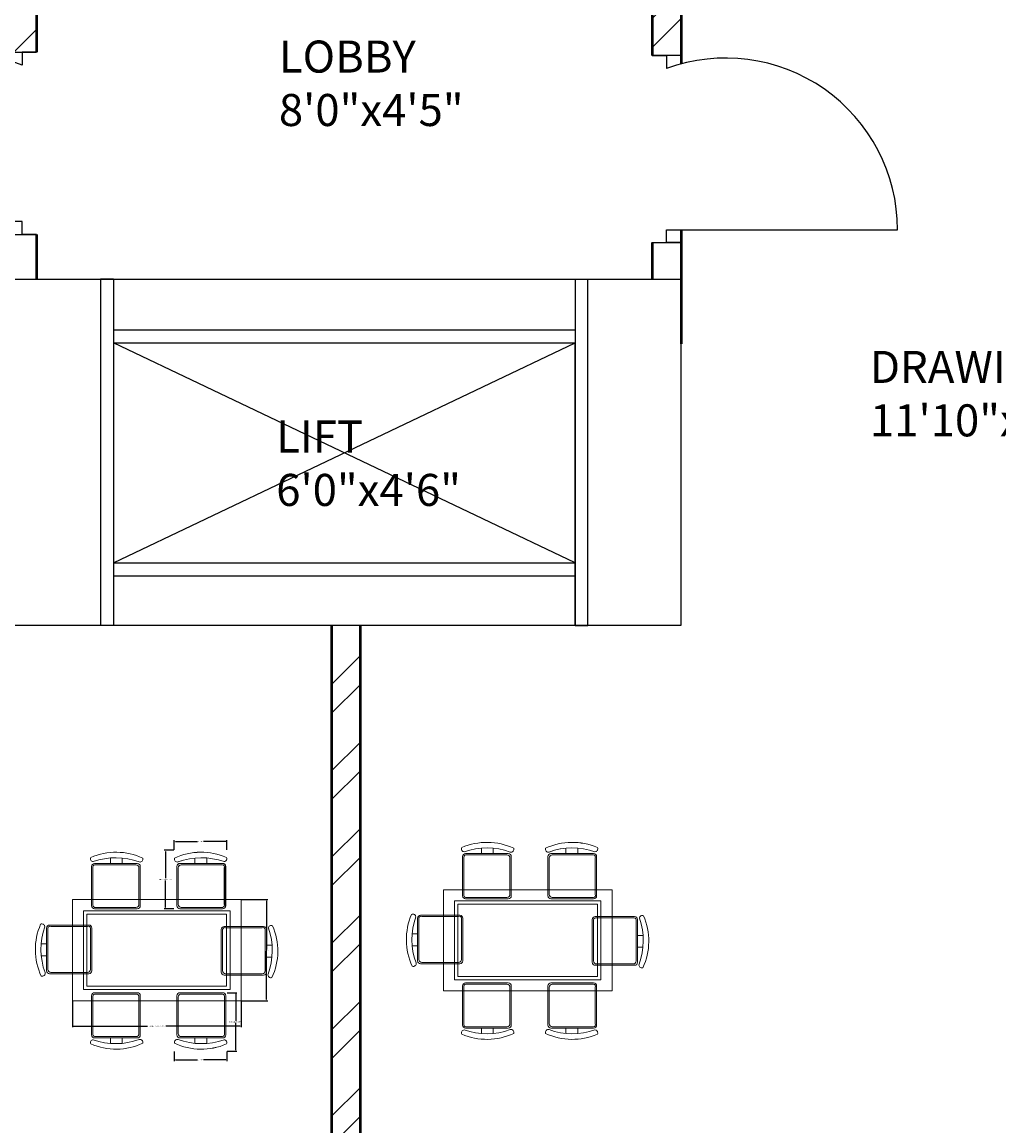
# Model space of a CAD drawing. Units: inches. Extents: x 2129 to 2642, y 1542 to 2414.
# Tile 7 of 9: x 2338 to 2490, y 2007 to 2179. Entities that reach past the tile are written whole.
import ezdxf

# ---------------------------------------------------------------- set-up
doc = ezdxf.new("R2010")
doc.units = ezdxf.units.IN
for name, color, linetype, lineweight in [('A-ANNO-DIMS', 2, 'Continuous', 18), ('A-AREA-IDEN', 7, 'Continuous', 18), ('A-DOOR', 3, 'Continuous', 25), ('A-FLOR-EVTR', 141, 'Continuous', 25), ('A-FURN', 8, 'Continuous', 18), ('A-WALL', 7, 'Continuous', 50), ('A-WALL-PATT', 252, 'Continuous', 13)]:
    doc.layers.add(name, color=color, linetype=linetype, lineweight=lineweight)
doc.styles.get("Standard").update_dxf_attribs({"font": 'arial.ttf'})
doc.dimstyles.get("Standard").update_dxf_attribs({"dimtxt": 0.18, "dimasz": 0.18, "dimexe": 0.18, "dimexo": 0.0625, "dimgap": 0.09, "dimtad": 0, "dimtih": 1, "dimtoh": 1, "dimdec": 4, "dimzin": 0, "dimdsep": 46, "dimtxsty": 'Standard', "dimcen": 0.09, "dimadec": 0, "dimazin": 0, "dimtfac": 1, "dimtdec": 4, "dimtofl": 0, "dimtmove": 0, "dimatfit": 3, "dimfxl": 1, "dimtolj": 1, "dimtzin": 0, "dimarcsym": 0})

# ---------------------------------------------------------------- blocks, each defined once
blk = doc.blocks.new('TABLE-DINING-RECT')
for points in [[(0, 15.8), (26.34, 15.8), (26.34, 0), (0, 0)], [(1.76, 14.05), (24.58, 14.05), (24.58, 1.76), (1.76, 1.76)], [(2.28, 13.52), (24.05, 13.52), (24.05, 2.28), (2.28, 2.28)]]:
    blk.add_lwpolyline(points, close=True)
blk = doc.blocks.new('CHAIR-DINING-SIDE')
for points in [[(7.53, 1.75, 0.414214), (8, 2.22), (8, 8.34, 0.414214), (7.53, 8.81), (0.87, 8.81, 0.414214), (0.4, 8.34), (0.4, 2.22, 0.414214), (0.87, 1.75), (7.53, 1.75)], [(3.21, 1.75), (3.21, 0.91, -0.064759)], [(7.74, 1.47, -0.175809), (0.57, 1.52, 0.578392), (0.02, 0.92, 0.214524), (8.12, 0.81, 0.552014), (7.74, 1.47, -0.065079)]]:
    blk.add_lwpolyline(points, format="xyb")
blk.add_lwpolyline([(7.53, 1.96), (1.08, 1.96, -0.414214), (0.61, 2.43), (0.61, 8.13, -0.414214), (1.08, 8.6), (7.53, 8.6, -0.512069), (7.79, 8.13), (7.79, 2.43, -0.512069)], format="xyb", close=True)
blk.add_lwpolyline([(5.07, 0.9), (5.07, 1.75)])
blk = doc.blocks.new('CHAIR-DINING-END')
for points in [[(0.57, 7.29, -0.578392), (0.02, 7.89, -0.214524), (8.12, 8, -0.552014), (7.74, 7.34, 0.175809), (0.57, 7.29)], [(7.53, 7.06, -0.414214), (8, 6.59), (8, 0.47, -0.414214), (7.53, 0), (0.87, 0, -0.414214), (0.4, 0.47), (0.4, 6.59, -0.414214), (0.87, 7.06), (7.53, 7.06)], [(3.21, 7.06), (3.21, 7.9, 0.064759)]]:
    blk.add_lwpolyline(points, format="xyb")
blk.add_lwpolyline([(5.07, 7.91), (5.07, 7.06)])
blk.add_lwpolyline([(7.53, 6.85), (1.08, 6.85, 0.414214), (0.61, 6.38), (0.61, 0.68, 0.414214), (1.08, 0.21), (7.53, 0.21, 0.512069), (7.79, 0.68), (7.79, 6.38, 0.512069)], format="xyb", close=True)
blk = doc.blocks.new('*D22')
at = {"layer": 'A-ANNO-DIMS', "color": 0, "lineweight": -2, "transparency": 16777216}
for p, q in [((2345.49, 2026.68), (2345.49, 2022.61)), ((2371.83, 2026.68), (2371.83, 2022.61)), ((2345.67, 2022.79), (2357.23, 2022.79)), ((2371.65, 2022.79), (2360.09, 2022.79))]:
    blk.add_line(p, q, dxfattribs=at)
at = {"layer": 'A-ANNO-DIMS', "color": 0, "transparency": 16777216}
for points in [[(2345.67, 2022.82), (2345.67, 2022.76), (2345.49, 2022.79)], [(2371.65, 2022.82), (2371.65, 2022.76), (2371.83, 2022.79)]]:
    blk.add_solid(points, dxfattribs=at)
at = {"layer": 'Defpoints', "color": 0, "transparency": 16777216}
for p in [(2345.49, 2026.74), (2371.83, 2026.74), (2371.83, 2022.79)]:
    blk.add_point(p, dxfattribs=at)
at = {"layer": 'A-ANNO-DIMS', "color": 0, "transparency": 16777216, "insert": (2358.66, 2022.79), "char_height": 0.18, "attachment_point": 5}
blk.add_mtext('\\A1;DINING TABLE 26 TYP.', dxfattribs=at)
blk = doc.blocks.new('*D23')
at = {"layer": 'A-ANNO-DIMS', "color": 0, "lineweight": -2, "transparency": 16777216}
for p, q in [((2371.89, 2042.54), (2375.96, 2042.54)), ((2375.78, 2042.36), (2375.78, 2034.82)), ((2375.78, 2026.92), (2375.78, 2034.46)), ((2371.89, 2026.74), (2375.96, 2026.74))]:
    blk.add_line(p, q, dxfattribs=at)
at = {"layer": 'A-ANNO-DIMS', "color": 0, "transparency": 16777216}
for points in [[(2375.75, 2042.36), (2375.81, 2042.36), (2375.78, 2042.54)], [(2375.75, 2026.92), (2375.81, 2026.92), (2375.78, 2026.74)]]:
    blk.add_solid(points, dxfattribs=at)
at = {"layer": 'Defpoints', "color": 0, "transparency": 16777216}
for p in [(2371.83, 2042.54), (2375.78, 2042.54), (2371.83, 2026.74)]:
    blk.add_point(p, dxfattribs=at)
at = {"layer": 'A-ANNO-DIMS', "color": 0, "transparency": 16777216, "insert": (2375.78, 2034.64), "char_height": 0.18, "attachment_point": 5}
blk.add_mtext('\\A1;16 TYP.', dxfattribs=at)
blk = doc.blocks.new('*D24')
at = {"layer": 'A-ANNO-DIMS', "color": 0, "lineweight": -2, "transparency": 16777216}
for p, q in [((2369.65, 2028), (2371.14, 2028)), ((2370.96, 2027.82), (2370.96, 2023.63)), ((2370.96, 2019.06), (2370.96, 2023.26)), ((2369.65, 2018.88), (2371.14, 2018.88))]:
    blk.add_line(p, q, dxfattribs=at)
at = {"layer": 'A-ANNO-DIMS', "color": 0, "transparency": 16777216}
for points in [[(2370.93, 2027.82), (2370.99, 2027.82), (2370.96, 2028)], [(2370.93, 2019.06), (2370.99, 2019.06), (2370.96, 2018.88)]]:
    blk.add_solid(points, dxfattribs=at)
at = {"layer": 'Defpoints', "color": 0, "transparency": 16777216}
for p in [(2369.59, 2028), (2370.96, 2028), (2369.59, 2018.88)]:
    blk.add_point(p, dxfattribs=at)
at = {"layer": 'A-ANNO-DIMS', "color": 0, "transparency": 16777216, "insert": (2370.96, 2023.44), "char_height": 0.18, "attachment_point": 5}
blk.add_mtext('\\A1;SIDE CHAIR 9 TYP.', dxfattribs=at)
blk = doc.blocks.new('*D25')
at = {"layer": 'A-ANNO-DIMS', "color": 0, "lineweight": -2, "transparency": 16777216}
for p, q in [((2361.37, 2018.82), (2361.37, 2017.34)), ((2369.59, 2018.82), (2369.59, 2017.34)), ((2361.55, 2017.52), (2365.02, 2017.52)), ((2369.41, 2017.52), (2365.94, 2017.52))]:
    blk.add_line(p, q, dxfattribs=at)
at = {"layer": 'A-ANNO-DIMS', "color": 0, "transparency": 16777216}
for points in [[(2361.55, 2017.55), (2361.55, 2017.49), (2361.37, 2017.52)], [(2369.41, 2017.55), (2369.41, 2017.49), (2369.59, 2017.52)]]:
    blk.add_solid(points, dxfattribs=at)
at = {"layer": 'Defpoints', "color": 0, "transparency": 16777216}
for p in [(2361.37, 2018.88), (2369.59, 2018.88), (2369.59, 2017.52)]:
    blk.add_point(p, dxfattribs=at)
at = {"layer": 'A-ANNO-DIMS', "color": 0, "transparency": 16777216, "insert": (2365.48, 2017.52), "char_height": 0.18, "attachment_point": 5}
blk.add_mtext('\\A1;8 TYP.', dxfattribs=at)
blk = doc.blocks.new('*D26')
at = {"layer": 'A-ANNO-DIMS', "color": 0, "lineweight": -2, "transparency": 16777216}
for p, q in [((2361.31, 2050.23), (2359.82, 2050.23)), ((2360, 2050.05), (2360, 2045.85)), ((2360, 2041.29), (2360, 2045.49)), ((2361.31, 2041.11), (2359.82, 2041.11))]:
    blk.add_line(p, q, dxfattribs=at)
at = {"layer": 'A-ANNO-DIMS', "color": 0, "transparency": 16777216}
for points in [[(2359.97, 2050.05), (2360.03, 2050.05), (2360, 2050.23)], [(2359.97, 2041.29), (2360.03, 2041.29), (2360, 2041.11)]]:
    blk.add_solid(points, dxfattribs=at)
at = {"layer": 'Defpoints', "color": 0, "transparency": 16777216}
for p in [(2360, 2050.23), (2361.37, 2050.23), (2361.37, 2041.11)]:
    blk.add_point(p, dxfattribs=at)
at = {"layer": 'A-ANNO-DIMS', "color": 0, "transparency": 16777216, "insert": (2360, 2045.67), "char_height": 0.18, "attachment_point": 5}
blk.add_mtext('\\A1;END CHAIR 9 TYP.', dxfattribs=at)
blk = doc.blocks.new('*D27')
at = {"layer": 'A-ANNO-DIMS', "color": 0, "lineweight": -2, "transparency": 16777216}
for p, q in [((2361.37, 2050.29), (2361.37, 2051.78)), ((2361.55, 2051.6), (2365.02, 2051.6)), ((2369.41, 2051.6), (2365.94, 2051.6)), ((2369.59, 2050.29), (2369.59, 2051.78))]:
    blk.add_line(p, q, dxfattribs=at)
at = {"layer": 'A-ANNO-DIMS', "color": 0, "transparency": 16777216}
for points in [[(2361.55, 2051.63), (2361.55, 2051.57), (2361.37, 2051.6)], [(2369.41, 2051.63), (2369.41, 2051.57), (2369.59, 2051.6)]]:
    blk.add_solid(points, dxfattribs=at)
at = {"layer": 'Defpoints', "color": 0, "transparency": 16777216}
for p in [(2369.59, 2051.6), (2361.37, 2050.23), (2369.59, 2050.23)]:
    blk.add_point(p, dxfattribs=at)
at = {"layer": 'A-ANNO-DIMS', "color": 0, "transparency": 16777216, "insert": (2365.48, 2051.6), "char_height": 0.18, "attachment_point": 5}
blk.add_mtext('\\A1;8 TYP.', dxfattribs=at)

msp = doc.modelspace()

# ---------------------------------------------------------------- hatches: boundary and pattern name
at = {"layer": 'A-WALL-PATT'}
h = msp.add_hatch(dxfattribs=at)
h.set_pattern_fill('ANSI32', color=256)
h.paths.add_polyline_path([(2306.2606, 2305.9717), (2306.2606, 2308.2217), (2276.3515, 2308.2217), (2276.3515, 2303.7217), (2306.2606, 2303.7217)])
h.paths.add_polyline_path([(2216.3515, 2305.9717), (2216.3515, 2308.2217), (2186.9043, 2308.2217), (2186.9043, 2278.1696), (2191.4043, 2278.1696), (2191.4043, 2303.7217), (2216.3515, 2303.7217)])
h.paths.add_polyline_path([(2339.9043, 2335.7217), (2362.1938, 2335.7217), (2362.1938, 2340.2217), (2335.4043, 2340.2217), (2335.4043, 2308.2217), (2329.3487, 2308.2217), (2329.3487, 2305.9717), (2329.3487, 2303.7217), (2335.4043, 2303.7217), (2335.4043, 2186.7217), (2329.4345, 2186.7217), (2329.4345, 2182.2217), (2335.4043, 2182.2217), (2335.4043, 2174.7178), (2339.9043, 2174.7178), (2339.9043, 2182.2217), (2339.9043, 2303.7217)])
h.paths.add_polyline_path([(2440.4043, 2340.2217), (2411.654, 2340.2217), (2411.654, 2335.7217), (2435.9043, 2335.7217), (2435.9043, 2303.7217), (2435.9043, 2182.2217), (2435.9043, 2174.1935), (2438.1543, 2174.1935), (2440.4043, 2174.1935), (2440.4043, 2182.2217), (2444.653, 2182.2217), (2444.653, 2184.4717), (2444.653, 2186.7217), (2440.4043, 2186.7217), (2440.4043, 2303.7217), (2445.8547, 2303.7217), (2445.8547, 2308.2217), (2440.4043, 2308.2217)])
h.paths.add_polyline_path([(2498.2381, 2308.2217), (2470.3901, 2308.2217), (2470.3901, 2303.7217), (2498.2381, 2303.7217), (2498.2381, 2305.9717)])
h.paths.add_polyline_path([(2588.9043, 2308.2217), (2586.9043, 2308.2217), (2558.2381, 2308.2217), (2558.2381, 2303.7217), (2584.4043, 2303.7217), (2584.4043, 2279.1087), (2588.9043, 2279.1087)])
h.paths.add_polyline_path([(2588.9043, 2219.1087), (2584.4043, 2219.1087), (2584.4043, 2186.7217), (2478.0667, 2186.7217), (2478.0667, 2182.2217), (2584.4043, 2182.2217), (2584.4043, 2157.7883), (2588.9043, 2157.7883)])
h.paths.add_polyline_path([(2588.9043, 2097.7883), (2584.6063, 2097.7883), (2584.6063, 2075.5462, -0.09241561), (2584.4043, 2074.4627), (2584.4043, 2064.2217), (2495.9043, 2064.2217), (2495.9043, 2040.4611), (2500.4043, 2040.4611), (2500.4043, 2059.7217), (2584.4043, 2059.7217), (2584.4043, 2052.2164), (2588.9043, 2052.2164)])
h.paths.add_polyline_path([(2588.9043, 2028.2164), (2584.4043, 2028.2164), (2584.4043, 2011.7217), (2500.4043, 2011.7217), (2500.4043, 2015.243), (2498.1543, 2015.243), (2495.9043, 2015.243), (2495.9043, 2007.2217), (2495.9043, 2003.7597), (2500.4043, 2003.7597), (2500.4043, 2007.2217), (2584.4043, 2007.2217), (2584.4043, 1992.1997), (2588.9043, 1992.1997)])
h.paths.add_polyline_path([(2588.9043, 1956.1997), (2584.4043, 1956.1997), (2584.4043, 1941.2217), (2500.4043, 1941.2217), (2500.4043, 1985.1493), (2498.1543, 1985.1493), (2495.9043, 1985.1493), (2495.9043, 1941.2217), (2435.9043, 1941.2217), (2435.9043, 1930.3963), (2440.4043, 1930.3963), (2440.4043, 1936.7217), (2584.4043, 1936.7217), (2584.4043, 1909.8406), (2588.9043, 1909.8406)])
h.paths.add_polyline_path([(2588.9043, 1849.8406), (2584.4043, 1849.8406), (2584.4043, 1801.3526), (2588.9043, 1801.3526)])
h.paths.add_polyline_path([(2584.4043, 1828.7217), (2495.9043, 1828.7217), (2440.4043, 1828.7217), (2440.4043, 1905.2159), (2438.1543, 1905.2159), (2435.9043, 1905.2159), (2435.9043, 1828.7217), (2428.9101, 1828.7217), (2428.9101, 1824.2217), (2584.4043, 1824.2217)])
h.paths.add_polyline_path([(2588.9043, 1741.3526), (2584.4043, 1741.3526), (2584.4043, 1704.2217), (2468.3173, 1704.2217), (2468.3173, 1701.9717), (2468.3173, 1699.7217), (2588.9043, 1699.7217)])
h.paths.add_polyline_path([(2442.4043, 1761.7217), (2435.0216, 1761.7217), (2435.0216, 1757.2217), (2437.9043, 1757.2217), (2437.9043, 1665.7217), (2442.4043, 1665.7217), (2442.4043, 1667.7217), (2442.4043, 1699.7217), (2446.6907, 1699.7217), (2446.6907, 1701.9717), (2446.6907, 1704.2217), (2442.4043, 1704.2217)])
h.paths.add_polyline_path([(2390.4043, 1757.2217), (2410.8996, 1757.2217), (2410.8996, 1761.7217), (2360.1741, 1761.7217), (2360.1741, 1759.4717), (2360.1741, 1757.2217), (2385.9043, 1757.2217), (2385.9043, 1674.8326), (2390.4043, 1674.8326)])
h.paths.add_polyline_path([(2337.9043, 1757.2217), (2340.3592, 1757.2217), (2340.3592, 1759.4717), (2340.3592, 1761.7217), (2333.4043, 1761.7217), (2333.4043, 1704.2217), (2327.381, 1704.2217), (2327.381, 1701.9717), (2327.381, 1699.7217), (2333.4043, 1699.7217), (2333.4043, 1665.7217), (2337.9043, 1665.7217)])
h.paths.add_polyline_path([(2191.4043, 1743.4804), (2186.9043, 1743.4804), (2186.9043, 1699.7217), (2188.9043, 1699.7217), (2191.4043, 1699.7217), (2306.5617, 1699.7217), (2306.5617, 1704.2217), (2191.4043, 1704.2217)])
h.paths.add_polyline_path([(2191.4043, 1859.8992), (2186.9043, 1859.8992), (2186.9043, 1803.4804), (2189.1543, 1803.4804), (2191.4043, 1803.4804)])
h.paths.add_polyline_path([(2352.5445, 1828.7217), (2191.4043, 1828.7217), (2191.4043, 1824.2217), (2333.4043, 1824.2217), (2352.5445, 1824.2217), (2352.5445, 1826.4717)])
h.paths.add_polyline_path([(2390.4043, 2085.328), (2385.9043, 2085.328), (2385.9043, 1828.7217), (2381.9668, 1828.7217), (2381.9668, 1826.4717), (2381.9668, 1824.2217), (2385.9043, 1824.2217), (2385.9043, 1761.7217), (2390.4043, 1761.7217), (2390.4043, 1824.2217), (2394.1868, 1824.2217), (2394.1868, 1827.6339), (2394.1868, 1828.7217), (2390.4043, 1828.7217)])
h.paths.add_polyline_path([(2339.9043, 1941.2217), (2335.4043, 1941.2217), (2279.9043, 1941.2217), (2279.9043, 1981.3432), (2277.6543, 1981.3432), (2275.4043, 1981.3432), (2275.4043, 1941.2217), (2191.4043, 1941.2217), (2191.4043, 1958.1079), (2186.9043, 1958.1079), (2186.9043, 1919.8992), (2189.1543, 1919.8992), (2191.4043, 1919.8992), (2191.4043, 1936.7217), (2279.9043, 1936.7217), (2335.4043, 1936.7217), (2335.4043, 1931.1382), (2339.9043, 1931.1382)])
h.paths.add_polyline_path([(2339.9043, 1902.7544), (2337.6543, 1902.7544), (2335.4043, 1902.7544), (2335.4043, 1828.7217), (2339.9043, 1828.7217)])
h.paths.add_polyline_path([(2279.9043, 2015.263), (2277.6543, 2015.263), (2275.4043, 2015.263), (2275.4043, 2011.7217), (2191.4043, 2011.7217), (2191.4043, 2026.6781), (2186.9043, 2026.6781), (2186.9043, 1994.1079), (2189.1543, 1994.1079), (2191.4043, 1994.1079), (2191.4043, 2007.2217), (2275.4043, 2007.2217), (2275.4043, 2003.2288), (2279.9043, 2003.2288), (2279.9043, 2007.2217)])
h.paths.add_polyline_path([(2296.0216, 2186.7217), (2191.4043, 2186.7217), (2191.4043, 2218.1696), (2186.9043, 2218.1696), (2186.9043, 2158.4509), (2191.4043, 2158.4509), (2191.4043, 2182.2217), (2296.0216, 2182.2217), (2296.0216, 2184.4717)])
h.paths.add_polyline_path([(2191.4043, 2098.4509), (2189.1543, 2098.4509), (2186.9043, 2098.4509), (2186.9043, 2050.6781), (2189.0487, 2050.6781), (2191.4043, 2050.6781), (2191.4043, 2059.7217), (2275.4043, 2059.7217), (2275.4043, 2038.4133), (2279.9043, 2038.4133), (2279.9043, 2064.2217), (2191.4043, 2064.2217)])
h.paths.add_polyline_path([(2268.3923, 1605.9386), (2516.3159, 1605.9386), (2516.3159, 1643.0314), (2268.3923, 1643.0314)], flags=9)
h.paths.add_polyline_path([(2399.6079, 1710.4489), (2428.8405, 1710.4489), (2428.8405, 1729.1062), (2399.6079, 1729.1062)], flags=9)
h.paths.add_polyline_path([(2342.1483, 1708.9956), (2371.3809, 1708.9956), (2371.3809, 1727.653), (2342.1483, 1727.653)], flags=9)
h.paths.add_polyline_path([(2200.7404, 1677.2519), (2282.3059, 1677.2519), (2282.3059, 1687.5555), (2200.7404, 1687.5555)], flags=9)
h.paths.add_polyline_path([(2209.8153, 1704.7448), (2250.627, 1704.7448), (2250.627, 1723.4021), (2209.8153, 1723.4021)], flags=25)
h.paths.add_polyline_path([(2213.9996, 1911.284), (2252.84, 1911.284), (2252.84, 1929.9413), (2213.9996, 1929.9413)], flags=9)
h.paths.add_polyline_path([(2210.8865, 1962.0987), (2244.0447, 1962.0987), (2244.0447, 1980.7561), (2210.8865, 1980.7561)], flags=25)
h.paths.add_polyline_path([(2219.0745, 2037.6131), (2248.2321, 2037.6131), (2248.2321, 2056.2705), (2219.0745, 2056.2705)], flags=9)
h.paths.add_polyline_path([(2379.9702, 2099.0686), (2409.3767, 2099.0686), (2409.3767, 2117.7259), (2379.9702, 2117.7259)], flags=9)
h.paths.add_polyline_path([(2375.9312, 2160.3752), (2405.3173, 2160.3752), (2405.3173, 2179.0325), (2375.9312, 2179.0325)], flags=9)
h.paths.add_polyline_path([(2269.5058, 2112.1824), (2310.3175, 2112.1824), (2310.3175, 2130.8397), (2269.5058, 2130.8397)], flags=9)
h.paths.add_polyline_path([(2209.6567, 2193.667), (2248.4971, 2193.667), (2248.4971, 2212.3243), (2209.6567, 2212.3243)], flags=25)
h.paths.add_polyline_path([(2491.6289, 1675.447), (2573.1944, 1675.447), (2573.1944, 1685.7506), (2491.6289, 1685.7506)], flags=9)
h.paths.add_polyline_path([(2492.0585, 1710.4489), (2530.8989, 1710.4489), (2530.8989, 1729.1062), (2492.0585, 1729.1062)], flags=25)
h.paths.add_polyline_path([(2495.6634, 1908.8646), (2534.5038, 1908.8646), (2534.5038, 1927.522), (2495.6634, 1927.522)], flags=9)
h.paths.add_polyline_path([(2516.7779, 1955.9942), (2549.9362, 1955.9942), (2549.9362, 1974.6516), (2516.7779, 1974.6516)], flags=25)
h.paths.add_polyline_path([(2509.7444, 2034.6896), (2538.902, 2034.6896), (2538.902, 2053.347), (2509.7444, 2053.347)], flags=9)
h.paths.add_polyline_path([(2467.8454, 2111.9593), (2508.6571, 2111.9593), (2508.6571, 2130.6167), (2467.8454, 2130.6167)], flags=9)
h.paths.add_polyline_path([(2528.5267, 2189.1742), (2567.3671, 2189.1742), (2567.3671, 2207.8316), (2528.5267, 2207.8316)], flags=25)
h.paths.add_polyline_path([(2483.7603, 2319.9841), (2557.5563, 2319.9841), (2557.5563, 2330.2877), (2483.7603, 2330.2877)], flags=9)
h.paths.add_polyline_path([(2204.078, 2317.0445), (2277.874, 2317.0445), (2277.874, 2327.3481), (2204.078, 2327.3481)], flags=9)

# ---------------------------------------------------------------- linework, layer by layer
at = {"layer": 'A-DOOR'}
for p, q in [((2335.4043, 2174.7178), (2339.9043, 2174.7178)), ((2339.9043, 2174.7178), (2337.6543, 2174.7178)), ((2337.6543, 2174.7178), (2337.6543, 2172.7178)), ((2440.4043, 2174.1935), (2435.9043, 2174.1935)), ((2435.9043, 2174.1935), (2438.1543, 2174.1935)), ((2438.1543, 2174.1935), (2438.1543, 2172.1935)), ((2337.6543, 2148.2947), (2301.6543, 2148.2947)), ((2337.6543, 2146.2947), (2337.6543, 2148.2947)), ((2335.4043, 2146.2947), (2339.9043, 2146.2947)), ((2339.9043, 2146.2947), (2337.6543, 2146.2947)), ((2438.1543, 2145.0357), (2438.1543, 2147.0357)), ((2438.1543, 2147.0357), (2474.1543, 2147.0357)), ((2435.9043, 2145.0357), (2440.4043, 2145.0357)), ((2440.4043, 2145.0357), (2438.1543, 2145.0357))]:
    msp.add_line(p, q, dxfattribs=at)
for centre, radius, start, end in [((2327.9389, 2148.2947), 26.2846, 68.307494, 180), ((2447.3639, 2147.0357), 26.7904, 0, 110.106306)]:
    msp.add_arc(centre, radius, start, end, dxfattribs=at)
at = {"layer": 'A-FLOR-EVTR'}
for p, q in [((2335.4043, 2139.328), (2440.4043, 2139.328)), ((2351.8875, 2139.328), (2349.8875, 2139.328)), ((2349.8875, 2139.328), (2349.8875, 2085.328)), ((2351.8875, 2139.328), (2351.8875, 2129.3885)), ((2423.9332, 2085.328), (2423.9332, 2139.328)), ((2423.9332, 2139.328), (2423.9332, 2139.328)), ((2425.8875, 2085.328), (2425.8875, 2139.328)), ((2440.4043, 2085.328), (2440.4043, 2139.328)), ((2423.9332, 2131.3885), (2351.8875, 2131.3885)), ((2351.8875, 2129.3885), (2423.8875, 2129.3885)), ((2423.8875, 2095.0441), (2351.8875, 2129.3885)), ((2351.8875, 2095.0441), (2423.8875, 2129.3885)), ((2351.8875, 2129.3885), (2351.8875, 2095.0441)), ((2423.8875, 2093.0441), (2423.8875, 2129.3885)), ((2423.8875, 2121.2821), (2423.8875, 2129.2217)), ((2425.8875, 2119.2821), (2425.8875, 2121.2821)), ((2351.8875, 2095.0441), (2423.8875, 2095.0441)), ((2351.8875, 2095.0441), (2351.8875, 2085.328)), ((2351.8875, 2093.0441), (2423.8875, 2093.0441)), ((2423.8875, 2085.2938), (2423.8875, 2093.0098)), ((2335.4043, 2085.328), (2440.4043, 2085.328)), ((2423.8875, 2085.2938), (2425.8875, 2085.2938))]:
    msp.add_line(p, q, dxfattribs=at)
at = {"layer": 'A-FURN'}
for points in [[(2406.5956, 2049.9924, -0.17580919), (2413.7691, 2049.9381, 0.57839206), (2414.3126, 2050.5356, 0.21452438), (2406.2152, 2050.6443, 0.55201397), (2406.5956, 2049.9924, -0.06507904)], [(2406.5956, 2049.9921, -0.17580919), (2413.7692, 2049.9378, 0.57839206), (2414.3126, 2050.5354, 0.21452438), (2406.2152, 2050.644, 0.55201397), (2406.5956, 2049.9921, -0.06507904)], [(2419.8084, 2049.9378, -0.57839206), (2419.2649, 2050.5354, -0.21452438), (2427.3623, 2050.644, -0.55201397), (2426.9819, 2049.9921, 0.1758092), (2419.8084, 2049.9378)], [(2348.7514, 2048.4556, -0.17580919), (2355.925, 2048.4013, 0.57839206), (2356.4684, 2048.9988, 0.21452438), (2348.371, 2049.1075, 0.55201397), (2348.7514, 2048.4556, -0.06507904)], [(2348.7514, 2048.4553, -0.17580919), (2355.925, 2048.401, 0.57839206), (2356.4684, 2048.9985, 0.21452438), (2348.371, 2049.1072, 0.55201397), (2348.7514, 2048.4553, -0.06507904)], [(2361.9642, 2048.4013, -0.57839206), (2361.4207, 2048.9988, -0.21452438), (2369.5181, 2049.1075, -0.55201397), (2369.1377, 2048.4556, 0.1758092), (2361.9642, 2048.4013)], [(2413.4648, 2049.7045), (2406.8051, 2049.7045, 0.41421356), (2406.3392, 2049.2386), (2406.3392, 2043.1151, 0.41421356), (2406.8051, 2042.6492), (2413.4648, 2042.6492, 0.41421356), (2413.9307, 2043.1151), (2413.9307, 2049.2386, 0.41421356), (2413.4648, 2049.7045)], [(2413.4648, 2049.7042), (2406.8051, 2049.7042, 0.41421356), (2406.3392, 2049.2383), (2406.3392, 2043.1148, 0.41421356), (2406.8051, 2042.6489), (2413.4648, 2042.6489, 0.41421356), (2413.9307, 2043.1148), (2413.9307, 2049.2383, 0.41421356), (2413.4648, 2049.7042)], [(2411.1256, 2049.7045), (2411.1256, 2050.5467, -0.06475861)], [(2411.1256, 2049.7042), (2411.1256, 2050.5464, -0.06475861)], [(2426.7724, 2049.7042, -0.41421356), (2427.2383, 2049.2383), (2427.2383, 2043.1148, -0.41421356), (2426.7724, 2042.6489), (2420.1127, 2042.6489, -0.41421356), (2419.6468, 2043.1148), (2419.6468, 2049.2383, -0.41421356), (2420.1127, 2049.7042), (2426.7724, 2049.7042)], [(2422.4519, 2049.7042), (2422.4519, 2050.5464, 0.06475861)], [(2355.6206, 2048.1677), (2348.961, 2048.1677, 0.41421356), (2348.495, 2047.7018), (2348.495, 2041.5783, 0.41421356), (2348.961, 2041.1124), (2355.6206, 2041.1124, 0.41421356), (2356.0865, 2041.5783), (2356.0865, 2047.7018, 0.41421356), (2355.6206, 2048.1677)], [(2355.6206, 2048.1674), (2348.961, 2048.1674, 0.41421356), (2348.495, 2047.7015), (2348.495, 2041.578, 0.41421356), (2348.961, 2041.1121), (2355.6206, 2041.1121, 0.41421356), (2356.0866, 2041.578), (2356.0866, 2047.7015, 0.41421356), (2355.6206, 2048.1674)], [(2353.2814, 2048.1677), (2353.2814, 2049.0099, -0.06475861)], [(2353.2814, 2048.1674), (2353.2814, 2049.0096, -0.06475861)], [(2368.9282, 2048.1677, -0.41421356), (2369.3941, 2047.7018), (2369.3941, 2041.5783, -0.41421356), (2368.9282, 2041.1124), (2362.2685, 2041.1124, -0.41421356), (2361.8026, 2041.5783), (2361.8026, 2047.7018, -0.41421356), (2362.2685, 2048.1677), (2368.9282, 2048.1677)], [(2364.6077, 2048.1677), (2364.6077, 2049.0099, 0.06475861)], [(2399.0907, 2032.6694, -0.57839206), (2398.4931, 2032.1259, -0.21452438), (2398.3845, 2040.2233, -0.55201397), (2399.0364, 2039.8429, 0.17580937), (2399.0907, 2032.6694)], [(2399.0907, 2032.6691, -0.57839206), (2398.4931, 2032.1256, -0.21452438), (2398.3845, 2040.2231, -0.55201397), (2399.0364, 2039.8426, 0.17580937), (2399.0907, 2032.6691)], [(2399.3243, 2039.6334, -0.41421356), (2399.7902, 2040.0993), (2405.9137, 2040.0993, -0.41421356), (2406.3796, 2039.6334), (2406.3796, 2032.9737, -0.41421356), (2405.9137, 2032.5078), (2399.7902, 2032.5078, -0.41421356), (2399.3243, 2032.9737), (2399.3243, 2039.6334)], [(2399.3243, 2039.6331, -0.41421356), (2399.7902, 2040.099), (2405.9137, 2040.099, -0.41421356), (2406.3796, 2039.6331), (2406.3796, 2032.9734, -0.41421356), (2405.9137, 2032.5075), (2399.7902, 2032.5075, -0.41421356), (2399.3243, 2032.9734), (2399.3243, 2039.6331)], [(2433.6185, 2039.4053, 0.41421356), (2433.1526, 2039.8712), (2427.0291, 2039.8712, 0.41421356), (2426.5632, 2039.4053), (2426.5632, 2032.7456, 0.41421356), (2427.0291, 2032.2797), (2433.1526, 2032.2797, 0.41421356), (2433.6185, 2032.7456), (2433.6185, 2039.4053)], [(2433.6185, 2039.405, 0.41421356), (2433.1526, 2039.871), (2427.0292, 2039.871, 0.41421356), (2426.5632, 2039.405), (2426.5632, 2032.7454, 0.41421356), (2427.0292, 2032.2794), (2433.1526, 2032.2794, 0.41421356), (2433.6185, 2032.7454), (2433.6185, 2039.405)], [(2433.9064, 2039.6148, -0.17580919), (2433.8521, 2032.4413, 0.57839206), (2434.4497, 2031.8978, 0.21452438), (2434.5583, 2039.9953, 0.55201397), (2433.9064, 2039.6148, -0.06507904)], [(2433.9064, 2039.6146, -0.17580919), (2433.8521, 2032.441, 0.57839206), (2434.4497, 2031.8976, 0.21452438), (2434.5583, 2039.995, 0.55201397), (2433.9064, 2039.6146, -0.06507904)], [(2341.2465, 2031.1326, -0.57839206), (2340.649, 2030.5891, -0.21452438), (2340.5403, 2038.6865, -0.55201397), (2341.1922, 2038.3061, 0.17580937), (2341.2465, 2031.1326)], [(2341.2465, 2031.1323, -0.57839206), (2340.649, 2030.5888, -0.21452438), (2340.5403, 2038.6862, -0.55201397), (2341.1922, 2038.3058, 0.17580937), (2341.2465, 2031.1323)], [(2341.4801, 2038.0966, -0.41421356), (2341.946, 2038.5625), (2348.0695, 2038.5625, -0.41421356), (2348.5354, 2038.0966), (2348.5354, 2031.4369, -0.41421356), (2348.0695, 2030.971), (2341.946, 2030.971, -0.41421356), (2341.4801, 2031.4369), (2341.4801, 2038.0966)], [(2341.4801, 2038.0963, -0.41421356), (2341.946, 2038.5622), (2348.0695, 2038.5622, -0.41421356), (2348.5354, 2038.0963), (2348.5354, 2031.4366, -0.41421356), (2348.0695, 2030.9707), (2341.946, 2030.9707, -0.41421356), (2341.4801, 2031.4366), (2341.4801, 2038.0963)], [(2375.7743, 2037.8685, 0.41421356), (2375.3084, 2038.3344), (2369.185, 2038.3344, 0.41421356), (2368.719, 2037.8685), (2368.719, 2031.2088, 0.41421356), (2369.185, 2030.7429), (2375.3084, 2030.7429, 0.41421356), (2375.7743, 2031.2088), (2375.7743, 2037.8685)], [(2375.7743, 2037.8682, 0.41421356), (2375.3084, 2038.3341), (2369.185, 2038.3341, 0.41421356), (2368.7191, 2037.8682), (2368.7191, 2031.2085, 0.41421356), (2369.185, 2030.7426), (2375.3084, 2030.7426, 0.41421356), (2375.7743, 2031.2085), (2375.7743, 2037.8682)], [(2376.0622, 2038.078, -0.17580919), (2376.0079, 2030.9045, 0.57839206), (2376.6055, 2030.361, 0.21452438), (2376.7141, 2038.4584, 0.55201397), (2376.0622, 2038.078, -0.06507904)], [(2376.0623, 2038.0777, -0.17580919), (2376.0079, 2030.9042, 0.57839206), (2376.6055, 2030.3608, 0.21452438), (2376.7141, 2038.4582, 0.55201397), (2376.0623, 2038.0778, -0.06507904)], [(2341.4801, 2033.7761), (2340.6379, 2033.7761, 0.06475861)], [(2341.4801, 2033.7758), (2340.6379, 2033.7758, 0.06475861)], [(2399.3243, 2035.3129), (2398.482, 2035.3129, 0.06475861)], [(2399.3243, 2035.3126), (2398.4821, 2035.3126, 0.06475861)], [(2433.6185, 2035.0848), (2434.4608, 2035.0848, -0.06475861)], [(2433.6185, 2035.0846), (2434.4608, 2035.0846, -0.06475861)], [(2375.7743, 2033.548), (2376.6166, 2033.548, -0.06475861)], [(2375.7743, 2033.5478), (2376.6166, 2033.5478, -0.06475861)], [(2413.4648, 2022.4843), (2406.8051, 2022.4843, -0.41421356), (2406.3392, 2022.9502), (2406.3392, 2029.0736, -0.41421356), (2406.8051, 2029.5396), (2413.4648, 2029.5396, -0.41421356), (2413.9307, 2029.0736), (2413.9307, 2022.9502, -0.41421356), (2413.4648, 2022.4843)], [(2413.4648, 2022.484), (2406.8051, 2022.484, -0.41421356), (2406.3392, 2022.9499), (2406.3392, 2029.0734, -0.41421356), (2406.8051, 2029.5393), (2413.4648, 2029.5393, -0.41421356), (2413.9307, 2029.0734), (2413.9307, 2022.9499, -0.41421356), (2413.4648, 2022.484)], [(2355.6206, 2020.9475), (2348.961, 2020.9475, -0.41421356), (2348.495, 2021.4134), (2348.495, 2027.5368, -0.41421356), (2348.961, 2028.0027), (2355.6206, 2028.0027, -0.41421356), (2356.0865, 2027.5368), (2356.0865, 2021.4134, -0.41421356), (2355.6206, 2020.9475)], [(2355.6206, 2020.9472), (2348.961, 2020.9472, -0.41421356), (2348.495, 2021.4131), (2348.495, 2027.5365, -0.41421356), (2348.961, 2028.0025), (2355.6206, 2028.0025, -0.41421356), (2356.0866, 2027.5365), (2356.0866, 2021.4131, -0.41421356), (2355.6206, 2020.9472)], [(2413.7691, 2022.2507, -0.57839206), (2414.3126, 2021.6531, -0.21452438), (2406.2152, 2021.5445, -0.55201397), (2406.5956, 2022.1964, 0.17580929), (2413.7691, 2022.2507)], [(2413.7692, 2022.2504, -0.57839206), (2414.3126, 2021.6528, -0.21452438), (2406.2152, 2021.5442, -0.55201397), (2406.5956, 2022.1961, 0.17580929), (2413.7692, 2022.2504)], [(2411.1256, 2022.4843), (2411.1256, 2021.642, 0.06475861)], [(2411.1256, 2022.484), (2411.1256, 2021.6418, 0.06475861)], [(2355.925, 2020.7139, -0.57839206), (2356.4684, 2020.1163, -0.21452438), (2348.371, 2020.0077, -0.55201397), (2348.7514, 2020.6596, 0.17580929), (2355.925, 2020.7139)], [(2355.925, 2020.7136, -0.57839206), (2356.4684, 2020.116, -0.21452438), (2348.371, 2020.0074, -0.55201397), (2348.7514, 2020.6593, 0.17580929), (2355.925, 2020.7136)], [(2353.2814, 2020.9475), (2353.2814, 2020.1052, 0.06475861)], [(2353.2814, 2020.9472), (2353.2814, 2020.1049, 0.06475861)]]:
    msp.add_lwpolyline(points, format="xyb", dxfattribs=at)
for points in [[(2406.808, 2049.4946), (2413.2549, 2049.4946, -0.41421356), (2413.7208, 2049.0287), (2413.7208, 2043.325, -0.41421356), (2413.2549, 2042.8591), (2406.808, 2042.8591, -0.51206948), (2406.5491, 2043.325), (2406.5491, 2049.0287, -0.51206948)], [(2406.808, 2049.4943), (2413.2549, 2049.4943, -0.41421356), (2413.7208, 2049.0284), (2413.7208, 2043.3247, -0.41421356), (2413.2549, 2042.8588), (2406.808, 2042.8588, -0.51206948), (2406.5491, 2043.3247), (2406.5491, 2049.0284, -0.51206948)], [(2426.7696, 2049.4943), (2420.3226, 2049.4943, 0.41421356), (2419.8567, 2049.0284), (2419.8567, 2043.3247, 0.41421356), (2420.3226, 2042.8588), (2426.7696, 2042.8588, 0.51206948), (2427.0284, 2043.3247), (2427.0284, 2049.0284, 0.51206948)], [(2348.9638, 2047.9578), (2355.4107, 2047.9578, -0.41421356), (2355.8766, 2047.4919), (2355.8766, 2041.7882, -0.41421356), (2355.4107, 2041.3223), (2348.9638, 2041.3223, -0.51206948), (2348.7049, 2041.7882), (2348.7049, 2047.4919, -0.51206948)], [(2348.9638, 2047.9575), (2355.4107, 2047.9575, -0.41421356), (2355.8767, 2047.4916), (2355.8767, 2041.7879, -0.41421356), (2355.4107, 2041.322), (2348.9638, 2041.322, -0.51206948), (2348.7049, 2041.7879), (2348.7049, 2047.4916, -0.51206948)], [(2368.9254, 2047.9578), (2362.4784, 2047.9578, 0.41421356), (2362.0125, 2047.4919), (2362.0125, 2041.7882, 0.41421356), (2362.4784, 2041.3223), (2368.9254, 2041.3223, 0.51206948), (2369.1842, 2041.7882), (2369.1842, 2047.4919, 0.51206948)], [(2399.5342, 2039.6306), (2399.5342, 2033.1836, 0.41421356), (2400.0001, 2032.7177), (2405.7038, 2032.7177, 0.41421356), (2406.1697, 2033.1836), (2406.1697, 2039.6306, 0.51206948), (2405.7038, 2039.8894), (2400.0001, 2039.8894, 0.51206948)], [(2399.5342, 2039.6303), (2399.5342, 2033.1833, 0.41421356), (2400.0001, 2032.7174), (2405.7038, 2032.7174, 0.41421356), (2406.1697, 2033.1833), (2406.1697, 2039.6303, 0.51206948), (2405.7038, 2039.8891), (2400.0001, 2039.8891, 0.51206948)], [(2433.4086, 2039.4025), (2433.4086, 2032.9555, -0.41421356), (2432.9427, 2032.4896), (2427.239, 2032.4896, -0.41421356), (2426.7731, 2032.9555), (2426.7731, 2039.4025, -0.51206948), (2427.239, 2039.6613), (2432.9427, 2039.6613, -0.51206948)], [(2433.4086, 2039.4022), (2433.4086, 2032.9553, -0.41421356), (2432.9427, 2032.4893), (2427.2391, 2032.4893, -0.41421356), (2426.7731, 2032.9553), (2426.7731, 2039.4022, -0.51206948), (2427.2391, 2039.6611), (2432.9427, 2039.6611, -0.51206948)], [(2341.69, 2038.0938), (2341.69, 2031.6468, 0.41421356), (2342.1559, 2031.1809), (2347.8596, 2031.1809, 0.41421356), (2348.3255, 2031.6468), (2348.3255, 2038.0938, 0.51206948), (2347.8596, 2038.3526), (2342.1559, 2038.3526, 0.51206948)], [(2341.69, 2038.0935), (2341.69, 2031.6465, 0.41421356), (2342.1559, 2031.1806), (2347.8596, 2031.1806, 0.41421356), (2348.3255, 2031.6465), (2348.3255, 2038.0935, 0.51206948), (2347.8596, 2038.3523), (2342.1559, 2038.3523, 0.51206948)], [(2375.5644, 2037.8657), (2375.5644, 2031.4187, -0.41421356), (2375.0985, 2030.9528), (2369.3949, 2030.9528, -0.41421356), (2368.9289, 2031.4187), (2368.9289, 2037.8657, -0.51206948), (2369.3949, 2038.1245), (2375.0985, 2038.1245, -0.51206948)], [(2375.5644, 2037.8654), (2375.5644, 2031.4184, -0.41421356), (2375.0985, 2030.9525), (2369.3949, 2030.9525, -0.41421356), (2368.929, 2031.4184), (2368.929, 2037.8654, -0.51206948), (2369.3949, 2038.1242), (2375.0985, 2038.1242, -0.51206948)], [(2406.808, 2022.6942), (2413.2549, 2022.6942, 0.41421356), (2413.7208, 2023.1601), (2413.7208, 2028.8637, 0.41421356), (2413.2549, 2029.3297), (2406.808, 2029.3297, 0.51206948), (2406.5491, 2028.8637), (2406.5491, 2023.1601, 0.51206948)], [(2406.808, 2022.6939), (2413.2549, 2022.6939, 0.41421356), (2413.7208, 2023.1598), (2413.7208, 2028.8635, 0.41421356), (2413.2549, 2029.3294), (2406.808, 2029.3294, 0.51206948), (2406.5491, 2028.8635), (2406.5491, 2023.1598, 0.51206948)], [(2348.9638, 2021.1574), (2355.4107, 2021.1574, 0.41421356), (2355.8766, 2021.6233), (2355.8766, 2027.3269, 0.41421356), (2355.4107, 2027.7928), (2348.9638, 2027.7928, 0.51206948), (2348.7049, 2027.3269), (2348.7049, 2021.6233, 0.51206948)], [(2348.9638, 2021.1571), (2355.4107, 2021.1571, 0.41421356), (2355.8767, 2021.623), (2355.8767, 2027.3266, 0.41421356), (2355.4107, 2027.7926), (2348.9638, 2027.7926, 0.51206948), (2348.7049, 2027.3266), (2348.7049, 2021.623, 0.51206948)]]:
    msp.add_lwpolyline(points, format="xyb", close=True, dxfattribs=at)
for points in [[(2409.2615, 2050.562), (2409.2615, 2049.7045)], [(2409.2615, 2050.5618), (2409.2615, 2049.7042)], [(2424.3161, 2050.5618), (2424.3161, 2049.7042)], [(2351.4173, 2049.0252), (2351.4173, 2048.1677)], [(2351.4173, 2049.0249), (2351.4173, 2048.1674)], [(2366.4719, 2049.0252), (2366.4719, 2048.1677)], [(2340.6226, 2035.6403), (2341.4801, 2035.6403)], [(2340.6226, 2035.64), (2341.4801, 2035.64)], [(2398.4667, 2037.1771), (2399.3243, 2037.1771)], [(2398.4668, 2037.1768), (2399.3243, 2037.1768)], [(2434.4761, 2036.949), (2433.6185, 2036.949)], [(2434.4761, 2036.9487), (2433.6185, 2036.9487)], [(2376.6319, 2035.4122), (2375.7743, 2035.4122)], [(2376.6319, 2035.4119), (2375.7743, 2035.4119)], [(2409.2615, 2021.6267), (2409.2615, 2022.4843)], [(2409.2615, 2021.6264), (2409.2615, 2022.484)], [(2351.4173, 2020.0899), (2351.4173, 2020.9475)], [(2351.4173, 2020.0896), (2351.4173, 2020.9472)]]:
    msp.add_lwpolyline(points, dxfattribs=at)
at = {"layer": 'A-WALL'}
for p, q in [((2339.9043, 2182.2217), (2339.9043, 2174.7178)), ((2435.9043, 2182.2217), (2435.9043, 2174.1935)), ((2440.4043, 2182.2217), (2440.4043, 2172.9064)), ((2339.9043, 2146.2947), (2339.9043, 2139.328)), ((2440.4043, 2147.0357), (2440.4043, 2129.2217)), ((2435.9043, 2145.0357), (2435.9043, 2139.328)), ((2385.9043, 2085.328), (2385.9043, 1828.7217)), ((2390.4043, 1828.7217), (2390.4043, 2085.328))]:
    msp.add_line(p, q, dxfattribs=at)

# ---------------------------------------------------------------- block references
at = {"layer": 'A-FURN'}
for name, p in [('CHAIR-DINING-END', (2419.2432, 2042.6491)), ('CHAIR-DINING-END', (2361.399, 2041.112)), ('TABLE-DINING-RECT', (2345.494, 2026.741)), ('TABLE-DINING-RECT', (2345.494, 2026.7407)), ('TABLE-DINING-RECT', (2403.3382, 2028.2778)), ('TABLE-DINING-RECT', (2403.3382, 2028.2775)), ('CHAIR-DINING-SIDE', (2419.2432, 2020.7298)), ('CHAIR-DINING-SIDE', (2419.2432, 2020.7295)), ('CHAIR-DINING-SIDE', (2361.399, 2019.193)), ('CHAIR-DINING-SIDE', (2361.399, 2019.1927))]:
    msp.add_blockref(name, p, dxfattribs=at)

# ---------------------------------------------------------------- texts
at = {"layer": 'A-AREA-IDEN', "char_height": 5, "attachment_point": 1}
for s, width, insert in [('LOBBY\\P8\'0"x4\'5"', 115.369897, (2377.6928, 2176.5479)), ('DRAWING\\P11\'10"x9\'10"', 102.911185, (2469.8559, 2128.1286)), ('LIFT\\P6\'0"x4\'6"', 60.250817, (2377.2811, 2117.2756))]:
    msp.add_mtext_dynamic_manual_height_columns(s, width=width, gutter_width=12.5, heights=[0], dxfattribs=dict(at, insert=insert))

# ---------------------------------------------------------------- dimensions: what is measured, and where the dimension line sits
at = {"layer": 'A-ANNO-DIMS'}
for base, p1, p2, text, picture, middle in [((2369.589, 2051.5985), (2361.3698, 2050.2307), (2369.589, 2050.2307), '<> TYP.', '*D27', (2365.4794, 2051.5985)), ((2371.8311, 2022.7904), (2345.4938, 2026.741), (2371.8311, 2026.741), 'DINING TABLE <> TYP.', '*D22', (2358.6624, 2022.7904)), ((2369.589, 2017.5164), (2361.3697, 2018.8841), (2369.589, 2018.8841), '<> TYP.', '*D25', (2365.4794, 2017.5164))]:
    dim = msp.add_linear_dim(base=base, p1=p1, p2=p2, text=text, dimstyle='Standard', override={"dimdec": 0, "dimlfac": 1, "dimrnd": 0, "dimzin": 0, "dimdsep": 46, "dimlunit": 2}, dxfattribs=at)
    dim.commit()
    dim.dimension.update_dxf_attribs({"geometry": picture, "text_midpoint": middle})
for base, p1, p2, text, picture, middle in [((2360.002, 2050.2307), (2361.3698, 2041.1121), (2361.3698, 2050.2307), 'END CHAIR <> TYP.', '*D26', (2360.002, 2045.6714)), ((2375.7817, 2042.5434), (2371.8311, 2026.741), (2371.8311, 2042.5434), '<> TYP.', '*D23', (2375.7817, 2034.6422)), ((2370.9568, 2028.0027), (2369.589, 2018.8841), (2369.589, 2028.0027), 'SIDE CHAIR <> TYP.', '*D24', (2370.9568, 2023.4434))]:
    dim = msp.add_linear_dim(base=base, p1=p1, p2=p2, angle=90, text=text, dimstyle='Standard', override={"dimdec": 0, "dimlfac": 1, "dimrnd": 0, "dimzin": 0, "dimdsep": 46, "dimlunit": 2}, dxfattribs=at)
    dim.commit()
    dim.dimension.update_dxf_attribs({"geometry": picture, "text_midpoint": middle})

doc.saveas('drawing.dxf')
